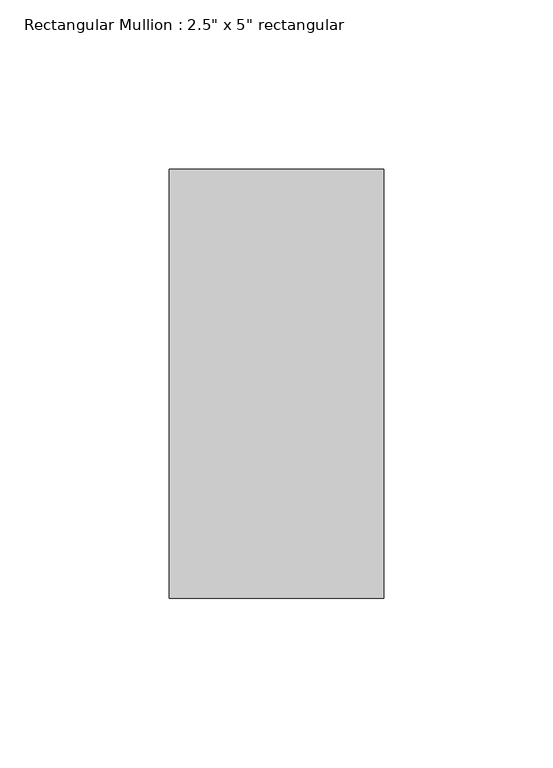
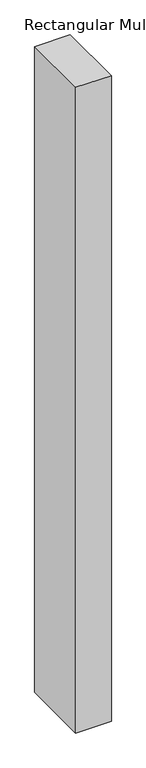
"""IFC4 building model written with IfcOpenShell, lengths in millimetres: member geometry."""

from ifc_helpers import new_model, si_unit, frame, origin, place, context, project, spatial, polyline, outline, extrude, source, transform, mapped, element, save


def member_2b49869a(model_context):
    return source(origin(), model_context, "Body", "SweptSolid", [
        extrude(outline(polyline([(31.75, 63.5), (31.75, -63.5), (-31.75, -63.5), (-31.75, 63.5), (31.75, 63.5)])), frame((0.0, 0.0, -1219.2), z_axis=(0.0, 0.0, 1.0), x_axis=(1.0, 0.0, 0.0)), (0.0, 0.0, 1.0), 1219.2),
    ])


if __name__ == "__main__":
    model = new_model("IFC4")
    model_context = context("Model", 3, world=origin())
    ifc_project = project(units=[si_unit("LENGTHUNIT", "METRE", prefix="MILLI")], contexts=[model_context])
    site = spatial("IfcSite", under=ifc_project)
    building = spatial("IfcBuilding", under=site)
    placement = place(None, origin())
    member_shape = member_2b49869a(model_context)
    element("IfcMember", 1, ObjectType="Rectangular Mullion : 2.5\" x 5\" rectangular", at=placement, inside=building, context=model_context, shape_type="MappedRepresentation", body=[
        mapped(member_shape, transform((0.0, 0.0, 0.0), x_axis=(1.0, 0.0, 0.0), y_axis=(0.0, 1.0, 0.0), z_axis=(0.0, 0.0, 1.0))),
    ])
    save(model, "model.ifc")

# Revit data of these elements
# Type "Rectangular Mullion : 2.5\" x 5\" rectangular"
#   built-in parameter 1007304 = 0.416667 (stored number, unit not read)
#   built-in parameter 1007301 = 0.104167 (stored number, unit not read)
#   built-in parameter 1007300 = 0.104167 (stored number, unit not read)
# Element 1 (IfcMember, "Rectangular Mullion : 2.5\" x 5\" rectangular")
#   Materials on its faces: "metal black"
# Materials
#   "metal black": class "Generic", colour RGB 120 120 120, transparency 0, Cost = 0
